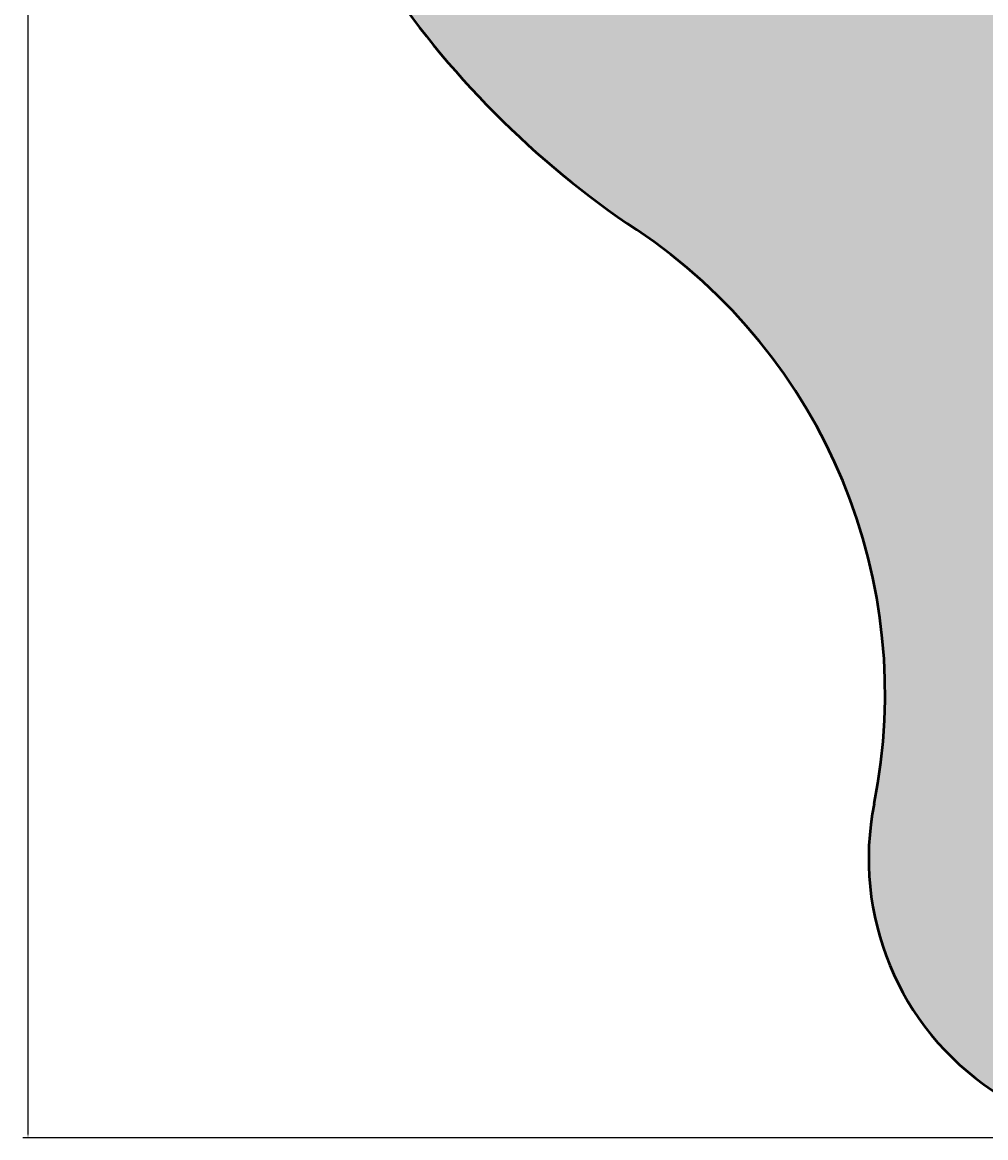
# Model space of a CAD drawing. Units: inches. Extents: x -13 to 107, y -48 to 102.
# Tile 1 of 13: x -13 to 22, y -47 to -7. Entities that reach past the tile are written whole.
import ezdxf

# ---------------------------------------------------------------- set-up
doc = ezdxf.new("R2010")
doc.units = ezdxf.units.IN
doc.header["$MEASUREMENT"] = 0
for name, color, linetype, lineweight in [('M-DIMS', 2, 'Continuous', 18), ('M-HATC', 8, 'Continuous', 18), ('M-OUTL', 7, 'Continuous', 50)]:
    doc.layers.add(name, color=color, linetype=linetype, lineweight=lineweight)
doc.styles.get("Standard").update_dxf_attribs({"font": 'arial.ttf'})
doc.dimstyles.get("Standard").update_dxf_attribs({"dimtxt": 0.18, "dimasz": 0.18, "dimexe": 0.18, "dimexo": 0.0625, "dimgap": 0.09, "dimtad": 0, "dimtih": 1, "dimtoh": 1, "dimdec": 4, "dimzin": 0, "dimdsep": 46, "dimtxsty": 'Standard', "dimcen": 0.09, "dimadec": 0, "dimazin": 0, "dimtfac": 1, "dimtdec": 4, "dimtofl": 0, "dimtmove": 0, "dimatfit": 3, "dimfxl": 1, "dimtolj": 1, "dimtzin": 0, "dimarcsym": 0})

# ---------------------------------------------------------------- blocks, each defined once
blk = doc.blocks.new('*D2')
at = {"layer": 'Defpoints', "color": 0, "transparency": 16777216}
for p in [(-12.585, 94.408), (27.547, 94.408), (27.547, -46.592)]:
    blk.add_point(p, dxfattribs=at)
at = {"layer": 'M-DIMS', "color": 0, "lineweight": -2, "transparency": 16777216}
for p, q in [((27.484, 94.408), (-12.765, 94.408)), ((-12.585, 94.228), (-12.585, 24.088)), ((-12.585, -46.412), (-12.585, 23.727)), ((27.484, -46.592), (-12.765, -46.592))]:
    blk.add_line(p, q, dxfattribs=at)
at = {"layer": 'M-DIMS', "color": 0, "transparency": 16777216}
for points in [[(-12.615, 94.228), (-12.555, 94.228), (-12.585, 94.408)], [(-12.615, -46.412), (-12.555, -46.412), (-12.585, -46.592)]]:
    blk.add_solid(points, dxfattribs=at)
at = {"layer": 'M-DIMS', "color": 0, "transparency": 16777216, "insert": (-12.585, 23.908), "char_height": 0.18, "attachment_point": 5}
blk.add_mtext('\\A1;141', dxfattribs=at)

msp = doc.modelspace()

# ---------------------------------------------------------------- hatches: boundary and pattern name
at = {"layer": 'M-HATC'}
h = msp.add_hatch(color=256, dxfattribs=at)
h.set_gradient(color1=(88, 186, 72), color2=(241, 235, 31), tint=1)
h.paths.add_polyline_path([(45.86, -14.044, 0.420873), (54.577, 32.339, -0.184081), (43.437, 76.537, 1.124637), (11.657, 76.537, -0.184081), (0.517, 32.339, 0.420873), (9.234, -14.044, -0.304084), (17.743, -34.622, 1.220926), (37.351, -34.622, -0.304084)])
h.paths.add_polyline_path([(33.479, -5.692, 0.859727), (21.615, -5.692, -0.111692), (13.972, -1.28, 0.859727), (8.04, 8.995, -0.111692), (8.04, 17.82, 0.859727), (13.972, 28.095, -0.111692), (21.615, 32.508, 0.859727), (33.479, 32.508, -0.111692), (41.122, 28.095, 0.859727), (47.054, 17.82, -0.111692), (47.054, 8.995, 0.859727), (41.122, -1.28, -0.111692)], flags=16)
h.paths.add_polyline_path([(32.547, -36.592, -1), (22.547, -36.592, -1)], flags=16)
h.paths.add_polyline_path([(17.547, 78.408, -1), (37.547, 78.408, -1)], flags=16)

# ---------------------------------------------------------------- linework, layer by layer
at = {"layer": 'M-OUTL'}
for centre, radius, start, end in [((27.547, 13.408), 33, 144.9933, 236.293), ((-1.865, -30.682), 20, 348.6384, 56.293), ((27.547, -36.592), 10, 168.6384, 11.3616)]:
    msp.add_arc(centre, radius, start, end, dxfattribs=at)

# ---------------------------------------------------------------- dimensions: what is measured, and where the dimension line sits
at = {"layer": 'M-DIMS'}
dim = msp.add_linear_dim(base=(-12.585, 94.408), p1=(27.547, -46.592), p2=(27.547, 94.408), angle=90, dimstyle='Standard', override={"dimdec": 0, "dimlfac": 1, "dimrnd": 0, "dimzin": 0, "dimdsep": 46, "dimlunit": 2}, dxfattribs=at)
dim.commit()
dim.dimension.update_dxf_attribs({"geometry": '*D2', "text_midpoint": (-12.585, 23.908)})

doc.saveas('drawing.dxf')
